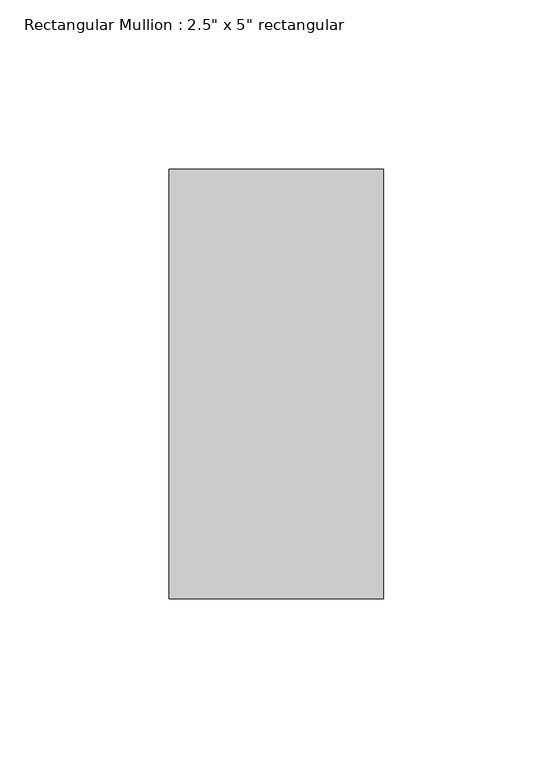
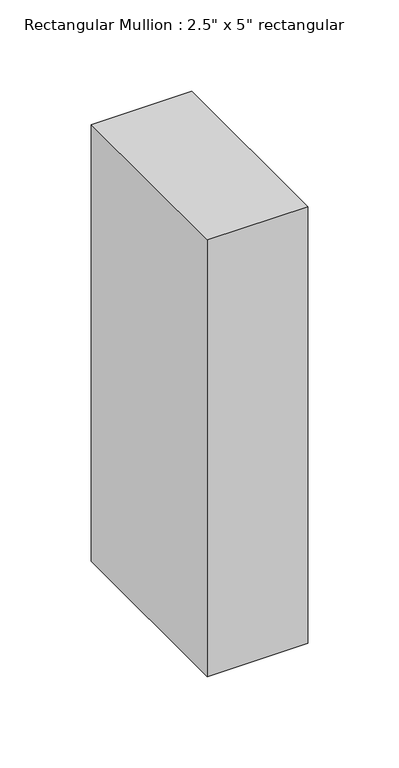
"""IFC4 building model written with IfcOpenShell, lengths in millimetres: member geometry."""

from ifc_helpers import new_model, si_unit, frame, origin, place, context, project, spatial, polyline, outline, extrude, source, transform, mapped, element, save


def member_177aa30a(model_context):
    return source(origin(), model_context, "Body", "SweptSolid", [
        extrude(outline(polyline([(0.0, 63.5), (0.0, -63.5), (-63.5, -63.5), (-63.5, 63.5), (0.0, 63.5)])), frame((0.0, 0.0, -292.1), z_axis=(0.0, 0.0, 1.0), x_axis=(1.0, 0.0, 0.0)), (0.0, 0.0, 1.0), 292.1),
    ])


if __name__ == "__main__":
    model = new_model("IFC4")
    model_context = context("Model", 3, world=origin())
    ifc_project = project(units=[si_unit("LENGTHUNIT", "METRE", prefix="MILLI")], contexts=[model_context])
    site = spatial("IfcSite", under=ifc_project)
    building = spatial("IfcBuilding", under=site)
    placement = place(None, origin())
    member_shape = member_177aa30a(model_context)
    element("IfcMember", 1, ObjectType="Rectangular Mullion : 2.5\" x 5\" rectangular", at=placement, inside=building, context=model_context, shape_type="MappedRepresentation", body=[
        mapped(member_shape, transform((0.0, 0.0, 0.0), x_axis=(1.0, 0.0, 0.0), y_axis=(0.0, 1.0, 0.0), z_axis=(0.0, 0.0, 1.0))),
    ])
    save(model, "model.ifc")

# Revit data of these elements
# Type "Rectangular Mullion : 2.5\" x 5\" rectangular"
#   built-in parameter 1007304 = 0.416667 (stored number, unit not read)
#   built-in parameter 1007301 = 0.104167 (stored number, unit not read)
#   built-in parameter 1007300 = 0.104167 (stored number, unit not read)
# Element 1 (IfcMember, "Rectangular Mullion : 2.5\" x 5\" rectangular")
#   Materials on its faces: "Aluminum"
# Materials
#   "Aluminum": class "Metal", colour RGB 247 247 247, transparency 0, Description = "Aluminum 6061", Cost = 0
